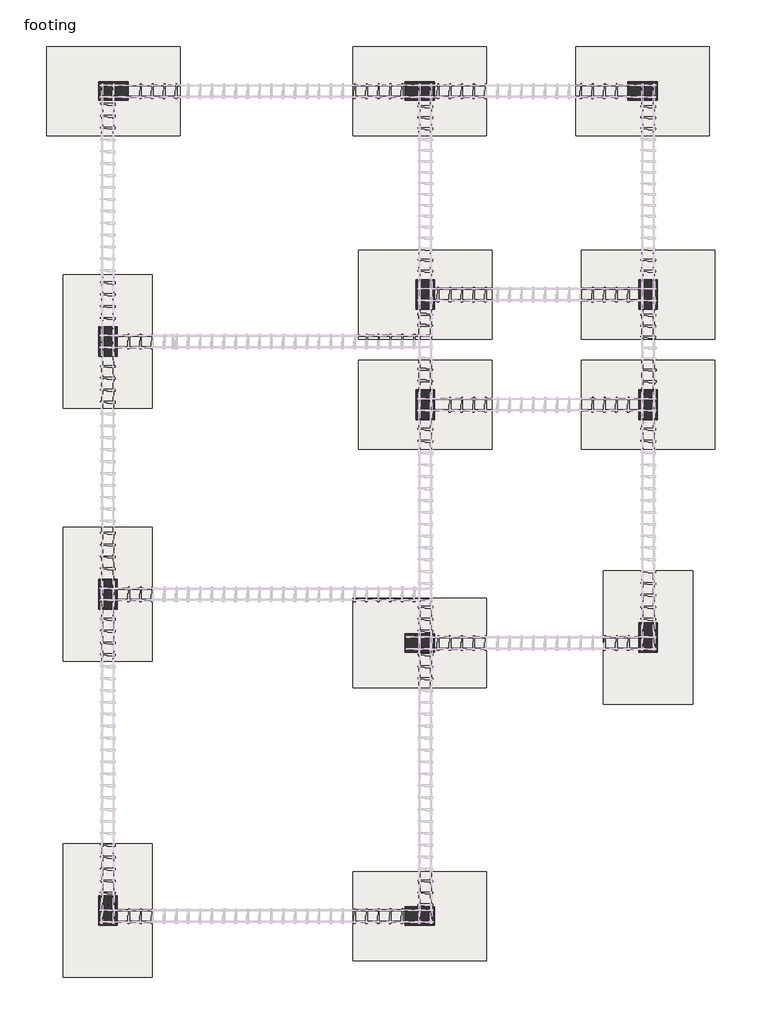
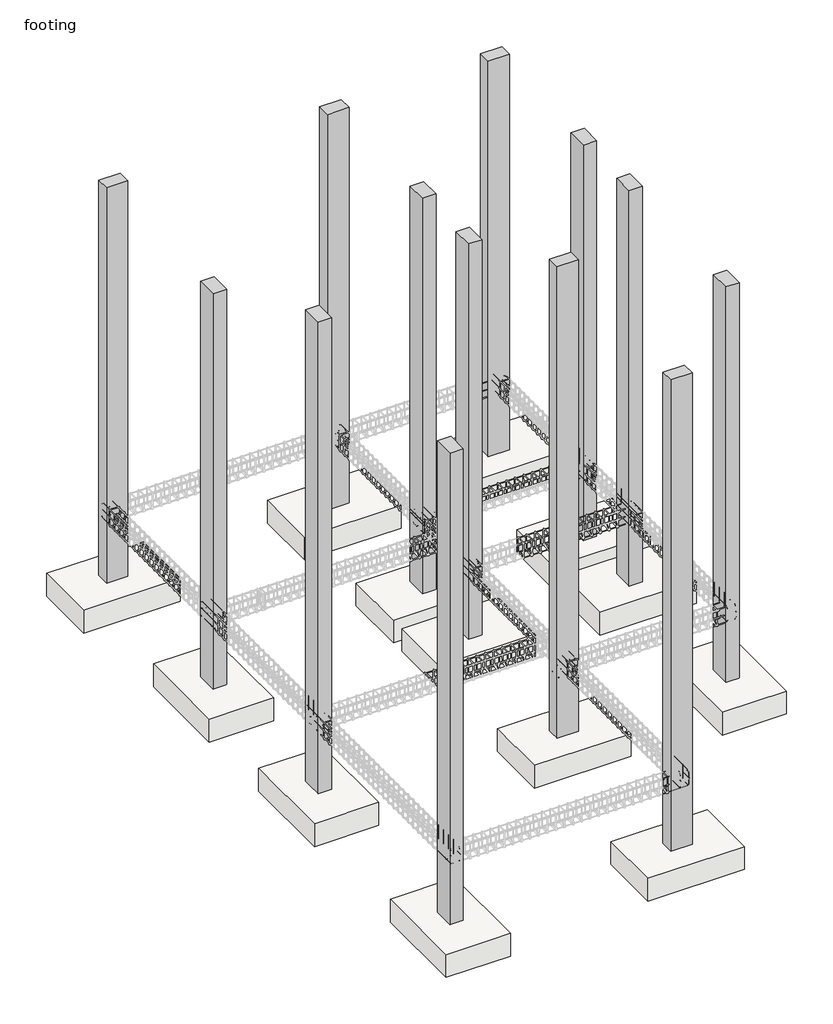
# One storey, part 1 of 21: 13 columns, 13 slabs.
"""IFC4 building model written with IfcOpenShell, lengths in millimetres."""

from ifc_helpers import new_model, si_unit, frame, origin, place, context, project, spatial, polyline, outline, extrude, transform, mapped, element, save
from components import footing_rectangular_footing_5ba74754

model = new_model("IFC4")

# Units and contexts
model_context = context("Model", 3, world=origin())
ifc_project = project(units=[si_unit("LENGTHUNIT", "METRE", prefix="MILLI")], contexts=[model_context])

# Site, building, storey
site = spatial("IfcSite", under=ifc_project)
building = spatial("IfcBuilding", under=site)
storey = spatial("IfcBuildingStorey", under=building, Name="footing", Elevation=-1524.0)

# Columns
placement = place(None, origin())
element("IfcColumn", 1, ObjectType="Concrete-Rectangular-Column : Column", at=placement, inside=storey, context=model_context, shape_type="SweptSolid", body=[
    extrude(outline(polyline([(-12336.5990423, 11108.5199494), (-11930.1990423, 11108.5199494), (-11930.1990423, 10854.5199494), (-12336.5990423, 10854.5199494), (-12336.5990423, 11108.5199494)])), frame((0.0, 0.0, -1524.0), z_axis=(0.0, 0.0, 1.0), x_axis=(1.0, 0.0, 0.0)), (0.0, 0.0, 1.0), 7924.8),
])
element("IfcColumn", 2, ObjectType="Concrete-Rectangular-Column : Column", at=placement, inside=storey, context=model_context, shape_type="SweptSolid", body=[
    extrude(outline(polyline([(-8145.5990423, 11108.5199494), (-7739.1990423, 11108.5199494), (-7739.1990423, 10854.5199494), (-8145.5990423, 10854.5199494), (-8145.5990423, 11108.5199494)])), frame((0.0, 0.0, -1524.0), z_axis=(0.0, 0.0, 1.0), x_axis=(1.0, 0.0, 0.0)), (0.0, 0.0, 1.0), 7924.8),
])
element("IfcColumn", 3, ObjectType="Concrete-Rectangular-Column : Column", at=placement, inside=storey, context=model_context, shape_type="SweptSolid", body=[
    extrude(outline(polyline([(-5097.5990423, 11108.5199494), (-4691.1990423, 11108.5199494), (-4691.1990423, 10854.5199494), (-5097.5990423, 10854.5199494), (-5097.5990423, 11108.5199494)])), frame((0.0, 0.0, -1524.0), z_axis=(0.0, 0.0, 1.0), x_axis=(1.0, 0.0, 0.0)), (0.0, 0.0, 1.0), 7924.8),
])
element("IfcColumn", 4, ObjectType="Concrete-Rectangular-Column : Column", at=placement, inside=storey, context=model_context, shape_type="SweptSolid", body=[
    extrude(outline(polyline([(-4945.1990423, 7997.0199494), (-4945.1990423, 8403.4199494), (-4691.1990423, 8403.4199494), (-4691.1990423, 7997.0199494), (-4945.1990423, 7997.0199494)])), frame((0.0, 0.0, -1524.0), z_axis=(0.0, 0.0, 1.0), x_axis=(1.0, 0.0, 0.0)), (0.0, 0.0, 1.0), 7924.8),
])
element("IfcColumn", 5, ObjectType="Concrete-Rectangular-Column : Column", at=placement, inside=storey, context=model_context, shape_type="SweptSolid", body=[
    extrude(outline(polyline([(-7739.1990423, 3310.7199494), (-8145.5990423, 3310.7199494), (-8145.5990423, 3564.7199494), (-7739.1990423, 3564.7199494), (-7739.1990423, 3310.7199494)])), frame((0.0, 0.0, -1524.0), z_axis=(0.0, 0.0, 1.0), x_axis=(1.0, 0.0, 0.0)), (0.0, 0.0, 1.0), 9448.8),
])
element("IfcColumn", 6, ObjectType="Concrete-Rectangular-Column : Column", at=placement, inside=storey, context=model_context, shape_type="SweptSolid", body=[
    extrude(outline(polyline([(-7993.1990423, 6492.0699494), (-7993.1990423, 6898.4699494), (-7739.1990423, 6898.4699494), (-7739.1990423, 6492.0699494), (-7993.1990423, 6492.0699494)])), frame((0.0, 0.0, -1524.0), z_axis=(0.0, 0.0, 1.0), x_axis=(1.0, 0.0, 0.0)), (0.0, 0.0, 1.0), 7924.8),
])
element("IfcColumn", 7, ObjectType="Concrete-Rectangular-Column : Column", at=placement, inside=storey, context=model_context, shape_type="SweptSolid", body=[
    extrude(outline(polyline([(-7993.1990423, 7997.0199494), (-7993.1990423, 8403.4199494), (-7739.1990423, 8403.4199494), (-7739.1990423, 7997.0199494), (-7993.1990423, 7997.0199494)])), frame((0.0, 0.0, -1524.0), z_axis=(0.0, 0.0, 1.0), x_axis=(1.0, 0.0, 0.0)), (0.0, 0.0, 1.0), 7924.8),
])
element("IfcColumn", 8, ObjectType="Concrete-Rectangular-Column : Column", at=placement, inside=storey, context=model_context, shape_type="SweptSolid", body=[
    extrude(outline(polyline([(-12336.5990423, 7355.6699494), (-12336.5990423, 7762.0699494), (-12082.5990423, 7762.0699494), (-12082.5990423, 7355.6699494), (-12336.5990423, 7355.6699494)])), frame((0.0, 0.0, -1524.0), z_axis=(0.0, 0.0, 1.0), x_axis=(1.0, 0.0, 0.0)), (0.0, 0.0, 1.0), 7924.8),
])
element("IfcColumn", 9, ObjectType="Concrete-Rectangular-Column : Column", at=placement, inside=storey, context=model_context, shape_type="SweptSolid", body=[
    extrude(outline(polyline([(-12336.5990423, 3901.2699494), (-12336.5990423, 4307.6699494), (-12082.5990423, 4307.6699494), (-12082.5990423, 3901.2699494), (-12336.5990423, 3901.2699494)])), frame((0.0, 0.0, -1524.0), z_axis=(0.0, 0.0, 1.0), x_axis=(1.0, 0.0, 0.0)), (0.0, 0.0, 1.0), 9448.8),
])
element("IfcColumn", 10, ObjectType="Concrete-Rectangular-Column : Column", at=placement, inside=storey, context=model_context, shape_type="SweptSolid", body=[
    extrude(outline(polyline([(-12336.5990423, -423.0800506), (-12336.5990423, -16.6800506), (-12082.5990423, -16.6800506), (-12082.5990423, -423.0800506), (-12336.5990423, -423.0800506)])), frame((0.0, 0.0, -1524.0), z_axis=(0.0, 0.0, 1.0), x_axis=(1.0, 0.0, 0.0)), (0.0, 0.0, 1.0), 9448.8),
])
element("IfcColumn", 11, ObjectType="Concrete-Rectangular-Column : Column", at=placement, inside=storey, context=model_context, shape_type="SweptSolid", body=[
    extrude(outline(polyline([(-7739.1990423, -423.0800506), (-8145.5990423, -423.0800506), (-8145.5990423, -169.0800506), (-7739.1990423, -169.0800506), (-7739.1990423, -423.0800506)])), frame((0.0, 0.0, -1524.0), z_axis=(0.0, 0.0, 1.0), x_axis=(1.0, 0.0, 0.0)), (0.0, 0.0, 1.0), 9448.8),
])
element("IfcColumn", 12, ObjectType="Concrete-Rectangular-Column : Column", at=placement, inside=storey, context=model_context, shape_type="SweptSolid", body=[
    extrude(outline(polyline([(-4691.1990423, 3717.1199494), (-4691.1990423, 3310.7199494), (-4945.1990423, 3310.7199494), (-4945.1990423, 3717.1199494), (-4691.1990423, 3717.1199494)])), frame((0.0, 0.0, -1524.0), z_axis=(0.0, 0.0, 1.0), x_axis=(1.0, 0.0, 0.0)), (0.0, 0.0, 1.0), 7924.8),
])
element("IfcColumn", 13, ObjectType="Concrete-Rectangular-Column : Column", at=placement, inside=storey, context=model_context, shape_type="SweptSolid", body=[
    extrude(outline(polyline([(-4691.1990423, 6898.4699494), (-4691.1990423, 6492.0699494), (-4945.1990423, 6492.0699494), (-4945.1990423, 6898.4699494), (-4691.1990423, 6898.4699494)])), frame((0.0, 0.0, -1524.0), z_axis=(0.0, 0.0, 1.0), x_axis=(1.0, 0.0, 0.0)), (0.0, 0.0, 1.0), 7924.8),
])

# Slabs
element("IfcSlab", 14, ObjectType="Footing-Rectangular : footing", at=placement, inside=storey, context=model_context, shape_type="SweptSolid", body=[
    extrude(outline(polyline([(-3903.7990423, 7590.6199494), (-5732.5990423, 7590.6199494), (-5732.5990423, 8809.8199494), (-3903.7990423, 8809.8199494), (-3903.7990423, 7590.6199494)])), frame((0.0, 0.0, -1981.2), z_axis=(0.0, 0.0, 1.0), x_axis=(1.0, 0.0, 0.0)), (0.0, 0.0, 1.0), 457.2),
])
element("IfcSlab", 15, ObjectType="Footing-Rectangular : footing", at=placement, inside=storey, context=model_context, shape_type="SweptSolid", body=[
    extrude(outline(polyline([(-3903.7990423, 6085.6699494), (-5732.5990423, 6085.6699494), (-5732.5990423, 7304.8699494), (-3903.7990423, 7304.8699494), (-3903.7990423, 6085.6699494)])), frame((0.0, 0.0, -1981.2), z_axis=(0.0, 0.0, 1.0), x_axis=(1.0, 0.0, 0.0)), (0.0, 0.0, 1.0), 457.2),
])
footing_rectangular_footing_shape = footing_rectangular_footing_5ba74754(model_context)
element("IfcSlab", 16, ObjectType="Footing-Rectangular : footing", at=placement, inside=storey, context=model_context, shape_type="MappedRepresentation", body=[
    mapped(footing_rectangular_footing_shape, transform((-12133.3990423, 10981.5199494, -1524.0), x_axis=(0.0, 1.0, 0.0), y_axis=(-1.0, 0.0, 0.0), z_axis=(0.0, 0.0, 1.0))),
])
element("IfcSlab", 17, ObjectType="Footing-Rectangular : footing", at=placement, inside=storey, context=model_context, shape_type="MappedRepresentation", body=[
    mapped(footing_rectangular_footing_shape, transform((-7942.3990423, 10981.5199494, -1524.0), x_axis=(0.0, 1.0, 0.0), y_axis=(-1.0, 0.0, 0.0), z_axis=(0.0, 0.0, 1.0))),
])
element("IfcSlab", 18, ObjectType="Footing-Rectangular : footing", at=placement, inside=storey, context=model_context, shape_type="MappedRepresentation", body=[
    mapped(footing_rectangular_footing_shape, transform((-4894.3990423, 10981.5199494, -1524.0), x_axis=(0.0, 1.0, 0.0), y_axis=(-1.0, 0.0, 0.0), z_axis=(0.0, 0.0, 1.0))),
])
element("IfcSlab", 19, ObjectType="Footing-Rectangular : footing", at=placement, inside=storey, context=model_context, shape_type="MappedRepresentation", body=[
    mapped(footing_rectangular_footing_shape, transform((-4818.1990423, 3513.9199494, -1524.0), x_axis=(1.0, 0.0, 0.0), y_axis=(0.0, 1.0, 0.0), z_axis=(0.0, 0.0, 1.0))),
])
element("IfcSlab", 20, ObjectType="Footing-Rectangular : footing", at=placement, inside=storey, context=model_context, shape_type="MappedRepresentation", body=[
    mapped(footing_rectangular_footing_shape, transform((-7942.3990423, 3437.7199494, -1524.0), x_axis=(0.0, 1.0, 0.0), y_axis=(-1.0, 0.0, 0.0), z_axis=(0.0, 0.0, 1.0))),
])
element("IfcSlab", 21, ObjectType="Footing-Rectangular : footing", at=placement, inside=storey, context=model_context, shape_type="MappedRepresentation", body=[
    mapped(footing_rectangular_footing_shape, transform((-7942.3990423, -296.0800506, -1524.0), x_axis=(0.0, 1.0, 0.0), y_axis=(-1.0, 0.0, 0.0), z_axis=(0.0, 0.0, 1.0))),
])
element("IfcSlab", 22, ObjectType="Footing-Rectangular : footing", at=placement, inside=storey, context=model_context, shape_type="MappedRepresentation", body=[
    mapped(footing_rectangular_footing_shape, transform((-12209.5990423, -219.8800506, -1524.0), x_axis=(-1.0, 0.0, 0.0), y_axis=(0.0, -1.0, 0.0), z_axis=(0.0, 0.0, 1.0))),
])
element("IfcSlab", 23, ObjectType="Footing-Rectangular : footing", at=placement, inside=storey, context=model_context, shape_type="MappedRepresentation", body=[
    mapped(footing_rectangular_footing_shape, transform((-12209.5990423, 4104.4699494, -1524.0), x_axis=(-1.0, 0.0, 0.0), y_axis=(0.0, -1.0, 0.0), z_axis=(0.0, 0.0, 1.0))),
])
element("IfcSlab", 24, ObjectType="Footing-Rectangular : footing", at=placement, inside=storey, context=model_context, shape_type="MappedRepresentation", body=[
    mapped(footing_rectangular_footing_shape, transform((-12209.5990423, 7558.8699494, -1524.0), x_axis=(-1.0, 0.0, 0.0), y_axis=(0.0, -1.0, 0.0), z_axis=(0.0, 0.0, 1.0))),
])
element("IfcSlab", 25, ObjectType="Footing-Rectangular : footing", at=placement, inside=storey, context=model_context, shape_type="MappedRepresentation", body=[
    mapped(footing_rectangular_footing_shape, transform((-7866.1990423, 6695.2699494, -1524.0), x_axis=(0.0, 1.0, 0.0), y_axis=(-1.0, 0.0, 0.0), z_axis=(0.0, 0.0, 1.0))),
])
element("IfcSlab", 26, ObjectType="Footing-Rectangular : footing", at=placement, inside=storey, context=model_context, shape_type="MappedRepresentation", body=[
    mapped(footing_rectangular_footing_shape, transform((-7866.1990423, 8200.2199494, -1524.0), x_axis=(0.0, 1.0, 0.0), y_axis=(-1.0, 0.0, 0.0), z_axis=(0.0, 0.0, 1.0))),
])

save(model, "model.ifc")

# Revit data of these elements
# Grids (mm)
#   "1": line (-1664.912, 10981.52) -> (-15311.837, 10981.52)
#   "2": line (-1664.912, 8200.22) -> (-15311.837, 8200.22)
#   "4": line (-1664.912, 6695.27) -> (-15311.837, 6695.27)
#   "6": line (-1664.912, 3437.72) -> (-15311.837, 3437.72)
#   "5": line (-1664.912, 4104.47) -> (-15311.837, 4104.47)
#   "7": line (-1664.912, -219.88) -> (-15311.837, -219.88)
#   "A": line (-12209.599, 13592.647) -> (-12209.599, -2803.102)
#   "B": line (-7942.399, 13592.647) -> (-7942.399, -2803.102)
#   "C": line (-4818.199, 13592.647) -> (-4818.199, -2803.102)
#   "3": line (-1664.912, 7558.87) -> (-15311.837, 7558.87)
# Type "Concrete-Rectangular-Column : Column"
#   Assembly Code = "B10"
#   b = 254 mm
#   h = 406.4 mm
#   Structural Material [instance default] = Concrete, Cast-in-Place gray
# Type "Footing-Rectangular : footing"
#   Assembly Code = "A1010100"
#   Width = 1219.2 mm
#   Length = 1828.8 mm
#   Foundation Thickness = 457.2 mm
#   Structural Material [instance default] = Concrete, Cast-in-Place gray
# Elements 1, 2, 3, 4, 5, 6, 7, 8, 9, 10, 11, 12, 13 (IfcColumn, "Concrete-Rectangular-Column : Column")
#   Structural Material = Concrete, Cast-in-Place gray
#   Phase Created = New Construction
#   Materials on its faces: "Concrete, Cast-in-Place gray"
# Elements 14, 15, 16, 17, 18, 19, 20, 21, 22, 23, 24, 25, 26 (IfcSlab, "Footing-Rectangular : footing")
#   Structural Material = Concrete, Cast-in-Place gray
#   Phase Created = New Construction
#   Materials on its faces: "Concrete, Cast-in-Place gray"
# Materials
#   "Concrete, Cast-in-Place gray": class "Concrete", colour RGB 192 192 192, transparency 0, Description = "Cast-in-place concrete", Cost = 0
